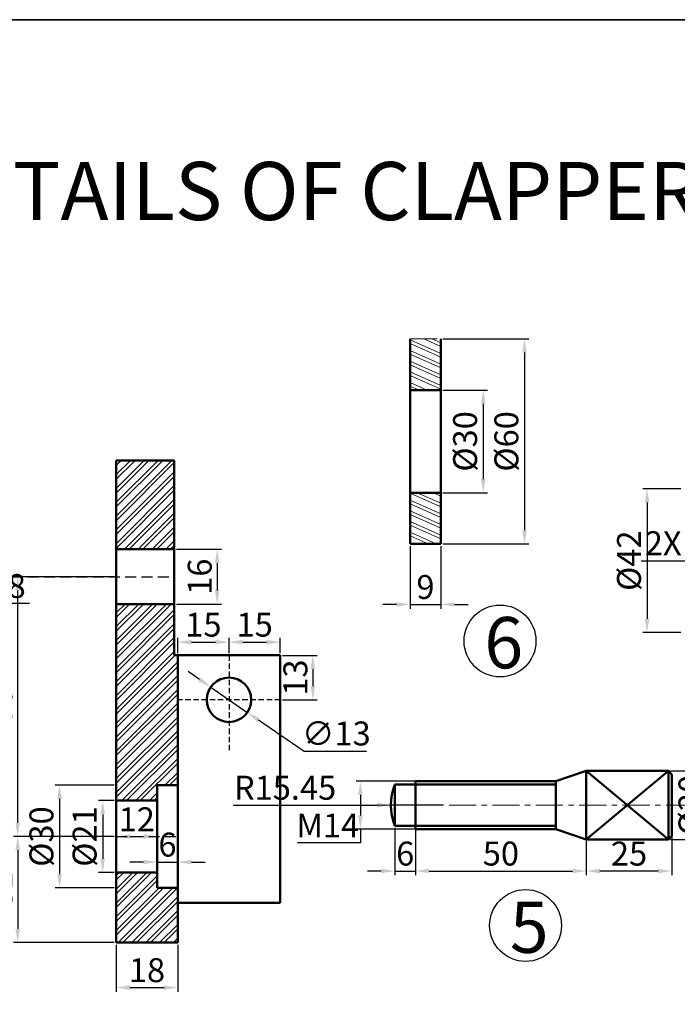
# Model space of a CAD drawing. Units: millimetres. Extents: x -108 to 732, y -172 to 297.
# Tile 3 of 4: x 91 to 284, y 9 to 297. Entities that reach past the tile are written whole.
import ezdxf

# ---------------------------------------------------------------- set-up
doc = ezdxf.new("R2010")
doc.units = ezdxf.units.MM
doc.header["$LTSCALE"] = 0.5
doc.linetypes.add('CENTER', pattern=[50.8, 31.75, -6.35, 6.35, -6.35])
doc.linetypes.add('HIDDEN', pattern=[9.525, 6.35, -3.175])
for name, color, linetype, lineweight in [('M-CNTR', 1, 'CENTER', 18), ('M-DIMS', 2, 'Continuous', 25), ('M-HATC', 8, 'Continuous', 18), ('M-HIDN', 6, 'HIDDEN', 25), ('M-OUTL', 7, 'Continuous', 50), ('M-SYMB', 3, 'Continuous', 25), ('M-TEXT', 3, 'Continuous', 25), ('M-TTLB', 7, 'Continuous', 35)]:
    doc.layers.add(name, color=color, linetype=linetype, lineweight=lineweight)
doc.styles.get("Standard").update_dxf_attribs({"font": 'arial.ttf'})
doc.dimstyles.new('ISO-25', dxfattribs={"dimtxt": 7, "dimasz": 4, "dimexe": 1.25, "dimexo": 0.625, "dimtad": 1, "dimtoh": 1, "dimtxsty": 'Standard', "dimcen": 2.5, "dimadec": 0, "dimazin": 0, "dimtfac": 1, "dimtmove": 0, "dimatfit": 3, "dimfxl": 1, "dimarcsym": 0})

# ---------------------------------------------------------------- blocks, each defined once
blk = doc.blocks.new('*D2')
at = {"layer": 'Defpoints', "color": 0, "ltscale": 0.5, "transparency": 16777216}
for p in [(119.6, 73.21), (103, 43.21), (119.6, 43.21)]:
    blk.add_point(p, dxfattribs=at)
at = {"layer": 'M-DIMS', "color": 0, "lineweight": -2, "ltscale": 0.5, "transparency": 16777216}
for p, q in [((118.97, 73.21), (101.75, 73.21)), ((103, 69.21), (103, 47.21)), ((118.97, 43.21), (101.75, 43.21))]:
    blk.add_line(p, q, dxfattribs=at)
at = {"layer": 'M-DIMS', "color": 0, "ltscale": 0.5, "transparency": 16777216}
for points in [[(102.33, 69.21), (103.67, 69.21), (103, 73.21)], [(102.33, 47.21), (103.67, 47.21), (103, 43.21)]]:
    blk.add_solid(points, dxfattribs=at)
at = {"layer": 'M-DIMS', "color": 0, "ltscale": 0.5, "transparency": 16777216, "insert": (98.61, 58.21), "char_height": 7, "attachment_point": 5, "rotation": 90}
blk.add_mtext('%%C30', dxfattribs=at)
blk = doc.blocks.new('*D3')
at = {"layer": 'Defpoints', "color": 0, "ltscale": 0.5, "transparency": 16777216}
for p in [(119.6, 68.71), (115.64, 47.71), (119.6, 47.71)]:
    blk.add_point(p, dxfattribs=at)
at = {"layer": 'M-DIMS', "color": 0, "lineweight": -2, "ltscale": 0.5, "transparency": 16777216}
for p, q in [((118.97, 68.71), (114.39, 68.71)), ((115.64, 64.71), (115.64, 51.71)), ((118.97, 47.71), (114.39, 47.71))]:
    blk.add_line(p, q, dxfattribs=at)
at = {"layer": 'M-DIMS', "color": 0, "ltscale": 0.5, "transparency": 16777216}
for points in [[(114.97, 64.71), (116.31, 64.71), (115.64, 68.71)], [(114.97, 51.71), (116.31, 51.71), (115.64, 47.71)]]:
    blk.add_solid(points, dxfattribs=at)
at = {"layer": 'M-DIMS', "color": 0, "ltscale": 0.5, "transparency": 16777216, "insert": (111.25, 58.21), "char_height": 7, "attachment_point": 5, "rotation": 90}
blk.add_mtext('%%C21', dxfattribs=at)
blk = doc.blocks.new('*D4')
at = {"layer": 'Defpoints', "color": 0, "ltscale": 0.5, "transparency": 16777216}
for p in [(152.6, 115.08), (137.6, 111.21), (152.6, 111.21)]:
    blk.add_point(p, dxfattribs=at)
at = {"layer": 'M-DIMS', "color": 0, "lineweight": -2, "ltscale": 0.5, "transparency": 16777216}
for p, q in [((137.6, 111.84), (137.6, 116.33)), ((152.6, 111.84), (152.6, 116.33)), ((141.6, 115.08), (148.6, 115.08))]:
    blk.add_line(p, q, dxfattribs=at)
at = {"layer": 'M-DIMS', "color": 0, "ltscale": 0.5, "transparency": 16777216}
for points in [[(141.6, 115.75), (141.6, 114.41), (137.6, 115.08)], [(148.6, 115.75), (148.6, 114.41), (152.6, 115.08)]]:
    blk.add_solid(points, dxfattribs=at)
at = {"layer": 'M-DIMS', "color": 0, "ltscale": 0.5, "transparency": 16777216, "insert": (145.1, 119.28), "char_height": 7, "attachment_point": 5}
blk.add_mtext('15', dxfattribs=at)
blk = doc.blocks.new('*D5')
at = {"layer": 'Defpoints', "color": 0, "ltscale": 0.5, "transparency": 16777216}
for p in [(167.6, 115.08), (152.6, 111.21), (167.6, 111.21)]:
    blk.add_point(p, dxfattribs=at)
at = {"layer": 'M-DIMS', "color": 0, "lineweight": -2, "ltscale": 0.5, "transparency": 16777216}
for p, q in [((152.6, 111.84), (152.6, 116.33)), ((167.6, 111.84), (167.6, 116.33)), ((156.6, 115.08), (163.6, 115.08))]:
    blk.add_line(p, q, dxfattribs=at)
at = {"layer": 'M-DIMS', "color": 0, "ltscale": 0.5, "transparency": 16777216}
for points in [[(156.6, 115.75), (156.6, 114.41), (152.6, 115.08)], [(163.6, 115.75), (163.6, 114.41), (167.6, 115.08)]]:
    blk.add_solid(points, dxfattribs=at)
at = {"layer": 'M-DIMS', "color": 0, "ltscale": 0.5, "transparency": 16777216, "insert": (160.1, 119.28), "char_height": 7, "attachment_point": 5}
blk.add_mtext('15', dxfattribs=at)
blk = doc.blocks.new('*D6')
at = {"layer": 'Defpoints', "color": 0, "ltscale": 0.5, "transparency": 16777216}
for p in [(167.6, 111.21), (167.6, 98.21), (177.13, 98.21)]:
    blk.add_point(p, dxfattribs=at)
at = {"layer": 'M-DIMS', "color": 0, "lineweight": -2, "ltscale": 0.5, "transparency": 16777216}
for p, q in [((168.22, 111.21), (178.38, 111.21)), ((177.13, 107.21), (177.13, 102.21)), ((168.22, 98.21), (178.38, 98.21))]:
    blk.add_line(p, q, dxfattribs=at)
at = {"layer": 'M-DIMS', "color": 0, "ltscale": 0.5, "transparency": 16777216}
for points in [[(176.46, 107.21), (177.8, 107.21), (177.13, 111.21)], [(176.46, 102.21), (177.8, 102.21), (177.13, 98.21)]]:
    blk.add_solid(points, dxfattribs=at)
at = {"layer": 'M-DIMS', "color": 0, "ltscale": 0.5, "transparency": 16777216, "insert": (172.93, 104.71), "char_height": 7, "attachment_point": 5, "rotation": 90}
blk.add_mtext('13', dxfattribs=at)
blk = doc.blocks.new('*D7')
at = {"layer": 'Defpoints', "color": 0, "ltscale": 0.5, "transparency": 16777216}
for p in [(119.6, 27.21), (137.6, 27.21), (137.6, 14.04)]:
    blk.add_point(p, dxfattribs=at)
at = {"layer": 'M-DIMS', "color": 0, "lineweight": -2, "ltscale": 0.5, "transparency": 16777216}
for p, q in [((119.6, 26.59), (119.6, 12.79)), ((137.6, 26.59), (137.6, 12.79)), ((123.6, 14.04), (133.6, 14.04))]:
    blk.add_line(p, q, dxfattribs=at)
at = {"layer": 'M-DIMS', "color": 0, "ltscale": 0.5, "transparency": 16777216}
for points in [[(123.6, 14.7), (123.6, 13.37), (119.6, 14.04)], [(133.6, 14.7), (133.6, 13.37), (137.6, 14.04)]]:
    blk.add_solid(points, dxfattribs=at)
at = {"layer": 'M-DIMS', "color": 0, "ltscale": 0.5, "transparency": 16777216, "insert": (128.6, 18.24), "char_height": 7, "attachment_point": 5}
blk.add_mtext('18', dxfattribs=at)
blk = doc.blocks.new('*D8')
at = {"layer": 'Defpoints', "color": 0, "ltscale": 0.5, "transparency": 16777216}
for p in [(137.6, 50.75), (131.6, 43.21), (137.6, 43.21)]:
    blk.add_point(p, dxfattribs=at)
at = {"layer": 'M-DIMS', "color": 0, "lineweight": -2, "ltscale": 0.5, "transparency": 16777216}
for p, q in [((131.6, 43.84), (131.6, 52)), ((137.6, 43.84), (137.6, 52)), ((127.6, 50.75), (123.6, 50.75)), ((131.6, 50.75), (137.6, 50.75)), ((141.6, 50.75), (145.6, 50.75))]:
    blk.add_line(p, q, dxfattribs=at)
at = {"layer": 'M-DIMS', "color": 0, "ltscale": 0.5, "transparency": 16777216}
for points in [[(127.6, 51.42), (127.6, 50.09), (131.6, 50.75)], [(141.6, 51.42), (141.6, 50.09), (137.6, 50.75)]]:
    blk.add_solid(points, dxfattribs=at)
at = {"layer": 'M-DIMS', "color": 0, "ltscale": 0.5, "transparency": 16777216, "insert": (134.6, 54.95), "char_height": 7, "attachment_point": 5}
blk.add_mtext('6', dxfattribs=at)
blk = doc.blocks.new('*D9')
at = {"layer": 'Defpoints', "color": 0, "ltscale": 0.5, "transparency": 16777216}
for p in [(119.6, 58.21), (90.76, 27.21), (119.6, 27.21)]:
    blk.add_point(p, dxfattribs=at)
at = {"layer": 'M-DIMS', "color": 0, "lineweight": -2, "ltscale": 0.5, "transparency": 16777216}
for p, q in [((118.97, 58.21), (89.51, 58.21)), ((90.76, 54.21), (90.76, 31.21)), ((118.97, 27.21), (89.51, 27.21))]:
    blk.add_line(p, q, dxfattribs=at)
at = {"layer": 'M-DIMS', "color": 0, "ltscale": 0.5, "transparency": 16777216}
for points in [[(90.09, 54.21), (91.43, 54.21), (90.76, 58.21)], [(90.09, 31.21), (91.43, 31.21), (90.76, 27.21)]]:
    blk.add_solid(points, dxfattribs=at)
at = {"layer": 'M-DIMS', "color": 0, "ltscale": 0.5, "transparency": 16777216, "insert": (86.56, 42.71), "char_height": 7, "attachment_point": 5, "rotation": 90}
blk.add_mtext('31', dxfattribs=at)
blk = doc.blocks.new('*D10')
at = {"layer": 'Defpoints', "color": 0, "ltscale": 0.5, "transparency": 16777216}
for p in [(90.76, 134.21), (119.6, 134.21), (90.76, 58.21)]:
    blk.add_point(p, dxfattribs=at)
at = {"layer": 'M-DIMS', "color": 0, "lineweight": -2, "ltscale": 0.5, "transparency": 16777216}
for p, q in [((118.97, 134.21), (89.51, 134.21)), ((90.76, 62.21), (90.76, 130.21)), ((90.14, 58.21), (89.51, 58.21))]:
    blk.add_line(p, q, dxfattribs=at)
at = {"layer": 'M-DIMS', "color": 0, "ltscale": 0.5, "transparency": 16777216}
for points in [[(90.09, 130.21), (91.43, 130.21), (90.76, 134.21)], [(90.09, 62.21), (91.43, 62.21), (90.76, 58.21)]]:
    blk.add_solid(points, dxfattribs=at)
at = {"layer": 'M-DIMS', "color": 0, "ltscale": 0.5, "transparency": 16777216, "insert": (86.56, 96.21), "char_height": 7, "attachment_point": 5, "rotation": 90}
blk.add_mtext('76', dxfattribs=at)
blk = doc.blocks.new('*D11')
at = {"layer": 'Defpoints', "color": 0, "ltscale": 0.5, "transparency": 16777216}
for p in [(147.25, 101.91), (157.95, 94.52)]:
    blk.add_point(p, dxfattribs=at)
at = {"layer": 'M-DIMS', "color": 0, "lineweight": -2, "ltscale": 0.5, "transparency": 16777216}
for p, q in [((143.96, 104.18), (140.67, 106.46)), ((147.25, 101.91), (157.95, 94.52)), ((174.55, 83.06), (161.24, 92.25)), ((192.81, 83.06), (174.55, 83.06))]:
    blk.add_line(p, q, dxfattribs=at)
at = {"layer": 'M-DIMS', "color": 0, "ltscale": 0.5, "transparency": 16777216}
for points in [[(144.34, 104.73), (143.58, 103.63), (147.25, 101.91)], [(161.62, 92.8), (160.86, 91.7), (157.95, 94.52)]]:
    blk.add_solid(points, dxfattribs=at)
at = {"layer": 'M-DIMS', "color": 0, "ltscale": 0.5, "transparency": 16777216, "insert": (183.99, 87.45), "char_height": 7, "attachment_point": 5}
blk.add_mtext('∅13', dxfattribs=at)
blk = doc.blocks.new('*D12')
at = {"layer": 'Defpoints', "color": 0, "ltscale": 0.5, "transparency": 16777216}
for p in [(136.6, 142.21), (136.6, 126.21), (149.14, 126.21)]:
    blk.add_point(p, dxfattribs=at)
at = {"layer": 'M-DIMS', "color": 0, "lineweight": -2, "ltscale": 0.5, "transparency": 16777216}
for p, q in [((137.22, 142.21), (150.39, 142.21)), ((149.14, 138.21), (149.14, 130.21)), ((137.22, 126.21), (150.39, 126.21))]:
    blk.add_line(p, q, dxfattribs=at)
at = {"layer": 'M-DIMS', "color": 0, "ltscale": 0.5, "transparency": 16777216}
for points in [[(148.47, 138.21), (149.8, 138.21), (149.14, 142.21)], [(148.47, 130.21), (149.8, 130.21), (149.14, 126.21)]]:
    blk.add_solid(points, dxfattribs=at)
at = {"layer": 'M-DIMS', "color": 0, "ltscale": 0.5, "transparency": 16777216, "insert": (144.94, 134.21), "char_height": 7, "attachment_point": 5, "rotation": 90}
blk.add_mtext('16', dxfattribs=at)
blk = doc.blocks.new('*D13')
at = {"layer": 'Defpoints', "color": 0, "ltscale": 0.5, "transparency": 16777216}
for p in [(119.6, 62.33), (131.6, 62.33), (131.6, 58.21)]:
    blk.add_point(p, dxfattribs=at)
at = {"layer": 'M-DIMS', "color": 0, "lineweight": -2, "ltscale": 0.5, "transparency": 16777216}
for p, q in [((119.6, 61.71), (119.6, 56.96)), ((131.6, 61.71), (131.6, 56.96)), ((123.6, 58.21), (127.6, 58.21))]:
    blk.add_line(p, q, dxfattribs=at)
at = {"layer": 'M-DIMS', "color": 0, "ltscale": 0.5, "transparency": 16777216}
for points in [[(123.6, 58.88), (123.6, 57.55), (119.6, 58.21)], [(127.6, 58.88), (127.6, 57.55), (131.6, 58.21)]]:
    blk.add_solid(points, dxfattribs=at)
at = {"layer": 'M-DIMS', "color": 0, "ltscale": 0.5, "transparency": 16777216, "insert": (125.6, 62.35), "char_height": 7, "attachment_point": 5}
blk.add_mtext('12', dxfattribs=at)
blk = doc.blocks.new('*D34')
at = {"layer": 'Defpoints', "color": 0, "ltscale": 0.5, "transparency": 16777216}
for p in [(214.58, 188.77), (214.58, 158.77), (226.99, 158.77)]:
    blk.add_point(p, dxfattribs=at)
at = {"layer": 'M-DIMS', "color": 0, "lineweight": -2, "ltscale": 0.5, "transparency": 16777216}
for p, q in [((215.2, 188.77), (228.24, 188.77)), ((226.99, 184.77), (226.99, 162.77)), ((215.2, 158.77), (228.24, 158.77))]:
    blk.add_line(p, q, dxfattribs=at)
at = {"layer": 'M-DIMS', "color": 0, "ltscale": 0.5, "transparency": 16777216}
for points in [[(226.32, 184.77), (227.65, 184.77), (226.99, 188.77)], [(226.32, 162.77), (227.65, 162.77), (226.99, 158.77)]]:
    blk.add_solid(points, dxfattribs=at)
at = {"layer": 'M-DIMS', "color": 0, "ltscale": 0.5, "transparency": 16777216, "insert": (222.59, 173.77), "char_height": 7, "attachment_point": 5, "rotation": 90}
blk.add_mtext('%%C30', dxfattribs=at)
blk = doc.blocks.new('*D35')
at = {"layer": 'Defpoints', "color": 0, "ltscale": 0.5, "transparency": 16777216}
for p in [(214.58, 203.77), (214.58, 143.77), (239.06, 143.77)]:
    blk.add_point(p, dxfattribs=at)
at = {"layer": 'M-DIMS', "color": 0, "lineweight": -2, "ltscale": 0.5, "transparency": 16777216}
for p, q in [((215.2, 203.77), (240.31, 203.77)), ((239.06, 199.77), (239.06, 147.77)), ((215.2, 143.77), (240.31, 143.77))]:
    blk.add_line(p, q, dxfattribs=at)
at = {"layer": 'M-DIMS', "color": 0, "ltscale": 0.5, "transparency": 16777216}
for points in [[(238.4, 199.77), (239.73, 199.77), (239.06, 203.77)], [(238.4, 147.77), (239.73, 147.77), (239.06, 143.77)]]:
    blk.add_solid(points, dxfattribs=at)
at = {"layer": 'M-DIMS', "color": 0, "ltscale": 0.5, "transparency": 16777216, "insert": (234.67, 173.77), "char_height": 7, "attachment_point": 5, "rotation": 90}
blk.add_mtext('%%C60', dxfattribs=at)
blk = doc.blocks.new('*D36')
at = {"layer": 'Defpoints', "color": 0, "ltscale": 0.5, "transparency": 16777216}
for p in [(205.58, 143.77), (214.58, 143.77), (214.58, 126.1)]:
    blk.add_point(p, dxfattribs=at)
at = {"layer": 'M-DIMS', "color": 0, "lineweight": -2, "ltscale": 0.5, "transparency": 16777216}
for p, q in [((205.58, 143.15), (205.58, 124.85)), ((214.58, 143.15), (214.58, 124.85)), ((201.58, 126.1), (197.58, 126.1)), ((205.58, 126.1), (214.58, 126.1)), ((218.58, 126.1), (222.58, 126.1))]:
    blk.add_line(p, q, dxfattribs=at)
at = {"layer": 'M-DIMS', "color": 0, "ltscale": 0.5, "transparency": 16777216}
for points in [[(201.58, 126.76), (201.58, 125.43), (205.58, 126.1)], [(218.58, 126.76), (218.58, 125.43), (214.58, 126.1)]]:
    blk.add_solid(points, dxfattribs=at)
at = {"layer": 'M-DIMS', "color": 0, "ltscale": 0.5, "transparency": 16777216, "insert": (210.08, 130.29), "char_height": 7, "attachment_point": 5}
blk.add_mtext('9', dxfattribs=at)
blk = doc.blocks.new('*D37')
at = {"layer": 'Defpoints', "color": 0, "ltscale": 0.5, "transparency": 16777216}
for p in [(201.16, 61.4), (207.16, 61.4), (207.16, 48.13)]:
    blk.add_point(p, dxfattribs=at)
at = {"layer": 'M-DIMS', "color": 0, "lineweight": -2, "ltscale": 0.5, "transparency": 16777216}
for p, q in [((201.16, 60.77), (201.16, 46.88)), ((207.16, 60.77), (207.16, 46.88)), ((197.16, 48.13), (193.16, 48.13)), ((201.16, 48.13), (207.16, 48.13)), ((211.16, 48.13), (215.16, 48.13))]:
    blk.add_line(p, q, dxfattribs=at)
at = {"layer": 'M-DIMS', "color": 0, "ltscale": 0.5, "transparency": 16777216}
for points in [[(197.16, 48.8), (197.16, 47.47), (201.16, 48.13)], [(211.16, 48.8), (211.16, 47.47), (207.16, 48.13)]]:
    blk.add_solid(points, dxfattribs=at)
at = {"layer": 'M-DIMS', "color": 0, "ltscale": 0.5, "transparency": 16777216, "insert": (204.16, 52.33), "char_height": 7, "attachment_point": 5}
blk.add_mtext('6', dxfattribs=at)
blk = doc.blocks.new('*D38')
at = {"layer": 'Defpoints', "color": 0, "ltscale": 0.5, "transparency": 16777216}
for p in [(207.16, 67.4), (257.16, 67.4), (257.16, 48.13)]:
    blk.add_point(p, dxfattribs=at)
at = {"layer": 'M-DIMS', "color": 0, "lineweight": -2, "ltscale": 0.5, "transparency": 16777216}
for p, q in [((207.16, 66.77), (207.16, 46.88)), ((257.16, 66.77), (257.16, 46.88)), ((211.16, 48.13), (253.16, 48.13))]:
    blk.add_line(p, q, dxfattribs=at)
at = {"layer": 'M-DIMS', "color": 0, "ltscale": 0.5, "transparency": 16777216}
for points in [[(211.16, 48.8), (211.16, 47.47), (207.16, 48.13)], [(253.16, 48.8), (253.16, 47.47), (257.16, 48.13)]]:
    blk.add_solid(points, dxfattribs=at)
at = {"layer": 'M-DIMS', "color": 0, "ltscale": 0.5, "transparency": 16777216, "insert": (232.16, 52.33), "char_height": 7, "attachment_point": 5}
blk.add_mtext('50', dxfattribs=at)
blk = doc.blocks.new('*D39')
at = {"layer": 'Defpoints', "color": 0, "ltscale": 0.5, "transparency": 16777216}
for p in [(257.16, 67.4), (282.16, 67.4), (257.16, 48.13)]:
    blk.add_point(p, dxfattribs=at)
at = {"layer": 'M-DIMS', "color": 0, "lineweight": -2, "ltscale": 0.5, "transparency": 16777216}
for p, q in [((257.16, 66.77), (257.16, 46.88)), ((282.16, 66.77), (282.16, 46.88)), ((278.16, 48.13), (261.16, 48.13))]:
    blk.add_line(p, q, dxfattribs=at)
at = {"layer": 'M-DIMS', "color": 0, "ltscale": 0.5, "transparency": 16777216}
for points in [[(261.16, 48.8), (261.16, 47.47), (257.16, 48.13)], [(278.16, 48.8), (278.16, 47.47), (282.16, 48.13)]]:
    blk.add_solid(points, dxfattribs=at)
at = {"layer": 'M-DIMS', "color": 0, "ltscale": 0.5, "transparency": 16777216, "insert": (269.66, 52.33), "char_height": 7, "attachment_point": 5}
blk.add_mtext('25', dxfattribs=at)
blk = doc.blocks.new('*D40')
at = {"layer": 'Defpoints', "color": 0, "ltscale": 0.5, "transparency": 16777216}
for p in [(281.16, 77.4), (281.16, 57.4), (292.93, 57.4)]:
    blk.add_point(p, dxfattribs=at)
at = {"layer": 'M-DIMS', "color": 0, "lineweight": -2, "ltscale": 0.5, "transparency": 16777216}
for p, q in [((281.79, 77.4), (294.18, 77.4)), ((292.93, 73.4), (292.93, 61.4)), ((281.79, 57.4), (294.18, 57.4))]:
    blk.add_line(p, q, dxfattribs=at)
at = {"layer": 'M-DIMS', "color": 0, "ltscale": 0.5, "transparency": 16777216}
for points in [[(292.26, 73.4), (293.59, 73.4), (292.93, 77.4)], [(292.26, 61.4), (293.59, 61.4), (292.93, 57.4)]]:
    blk.add_solid(points, dxfattribs=at)
at = {"layer": 'M-DIMS', "color": 0, "ltscale": 0.5, "transparency": 16777216, "insert": (288.53, 67.4), "char_height": 7, "attachment_point": 5, "rotation": 90}
blk.add_mtext('%%C20', dxfattribs=at)
blk = doc.blocks.new('*D41')
at = {"layer": 'Defpoints', "color": 0, "ltscale": 0.5, "transparency": 16777216}
for p in [(212.85, 74.4), (191.05, 60.4), (212.85, 60.4)]:
    blk.add_point(p, dxfattribs=at)
at = {"layer": 'M-DIMS', "color": 0, "lineweight": -2, "ltscale": 0.5, "transparency": 16777216}
for p, q in [((212.23, 74.4), (189.8, 74.4)), ((191.05, 70.4), (191.05, 64.4)), ((212.23, 60.4), (189.8, 60.4)), ((191.05, 60.4), (191.05, 56.4)), ((191.05, 56.4), (172.6, 56.4))]:
    blk.add_line(p, q, dxfattribs=at)
at = {"layer": 'M-DIMS', "color": 0, "ltscale": 0.5, "transparency": 16777216}
for points in [[(190.38, 70.4), (191.71, 70.4), (191.05, 74.4)], [(190.38, 64.4), (191.71, 64.4), (191.05, 60.4)]]:
    blk.add_solid(points, dxfattribs=at)
at = {"layer": 'M-DIMS', "color": 0, "ltscale": 0.5, "transparency": 16777216, "insert": (181.51, 60.54), "char_height": 7, "attachment_point": 5}
blk.add_mtext('M14', dxfattribs=at)
blk = doc.blocks.new('*D46')
at = {"layer": 'Defpoints', "color": 0, "ltscale": 0.5, "transparency": 16777216}
for p in [(285.41, 159.89), (274.94, 117.89), (285.41, 117.89)]:
    blk.add_point(p, dxfattribs=at)
at = {"layer": 'M-DIMS', "color": 0, "lineweight": -2, "ltscale": 0.5, "transparency": 16777216}
for p, q in [((284.79, 159.89), (273.69, 159.89)), ((274.94, 155.89), (274.94, 121.89)), ((284.79, 117.89), (273.69, 117.89))]:
    blk.add_line(p, q, dxfattribs=at)
at = {"layer": 'M-DIMS', "color": 0, "ltscale": 0.5, "transparency": 16777216}
for points in [[(274.28, 155.89), (275.61, 155.89), (274.94, 159.89)], [(274.28, 121.89), (275.61, 121.89), (274.94, 117.89)]]:
    blk.add_solid(points, dxfattribs=at)
at = {"layer": 'M-DIMS', "color": 0, "ltscale": 0.5, "transparency": 16777216, "insert": (270.55, 138.89), "char_height": 7, "attachment_point": 5, "rotation": 90}
blk.add_mtext('%%C42', dxfattribs=at)
blk = doc.blocks.new('*D54')
at = {"layer": 'Defpoints', "color": 0, "ltscale": 0.5, "transparency": 16777216}
for p in [(45.34, 134.21), (52.87, 131.51)]:
    blk.add_point(p, dxfattribs=at)
at = {"layer": 'M-DIMS', "color": 0, "lineweight": -2, "ltscale": 0.5, "transparency": 16777216}
for p, q in [((45.34, 134.21), (52.87, 131.51)), ((67.12, 126.38), (56.63, 130.15)), ((94.21, 126.38), (67.12, 126.38))]:
    blk.add_line(p, q, dxfattribs=at)
at = {"layer": 'M-DIMS', "color": 0, "ltscale": 0.5, "transparency": 16777216}
blk.add_solid([(56.86, 130.78), (56.41, 129.53), (52.87, 131.51)], dxfattribs=at)
at = {"layer": 'M-DIMS', "color": 0, "ltscale": 0.5, "transparency": 16777216, "insert": (80.98, 130.58), "char_height": 7, "attachment_point": 5}
blk.add_mtext('2X R8', dxfattribs=at)
blk = doc.blocks.new('*D59')
at = {"layer": 'Defpoints', "color": 0, "ltscale": 0.5, "transparency": 16777216}
for p in [(315.41, 138.89), (324.41, 138.89)]:
    blk.add_point(p, dxfattribs=at)
at = {"layer": 'M-DIMS', "color": 0, "lineweight": -2, "ltscale": 0.5, "transparency": 16777216}
for p, q in [((273.18, 138.89), (300.26, 138.89)), ((300.26, 138.89), (311.41, 138.89)), ((324.41, 138.89), (315.41, 138.89))]:
    blk.add_line(p, q, dxfattribs=at)
at = {"layer": 'M-DIMS', "color": 0, "ltscale": 0.5, "transparency": 16777216}
blk.add_solid([(311.41, 139.56), (311.41, 138.23), (315.41, 138.89)], dxfattribs=at)
at = {"layer": 'M-DIMS', "color": 0, "ltscale": 0.5, "transparency": 16777216, "insert": (286.41, 143.09), "char_height": 7, "attachment_point": 5}
blk.add_mtext('2X R9', dxfattribs=at)
blk = doc.blocks.new('*D60')
at = {"layer": 'Defpoints', "color": 0, "ltscale": 0.5, "transparency": 16777216}
for p in [(199.95, 67.4), (215.4, 67.4)]:
    blk.add_point(p, dxfattribs=at)
at = {"layer": 'M-DIMS', "color": 0, "lineweight": -2, "ltscale": 0.5, "transparency": 16777216}
for p, q in [((153.8, 67.4), (184.8, 67.4)), ((184.8, 67.4), (195.95, 67.4)), ((215.4, 67.4), (199.95, 67.4))]:
    blk.add_line(p, q, dxfattribs=at)
at = {"layer": 'M-DIMS', "color": 0, "ltscale": 0.5, "transparency": 16777216}
blk.add_solid([(195.95, 68.06), (195.95, 66.73), (199.95, 67.4)], dxfattribs=at)
at = {"layer": 'M-DIMS', "color": 0, "ltscale": 0.5, "transparency": 16777216, "insert": (168.99, 71.59), "char_height": 7, "attachment_point": 5}
blk.add_mtext('R15.45', dxfattribs=at)

msp = doc.modelspace()

# ---------------------------------------------------------------- hatches: boundary and pattern name
at = {"layer": 'M-HATC', "ltscale": 0.5}
h = msp.add_hatch(dxfattribs=at)
h.set_pattern_fill('ANSI32', color=256, scale=0.3, angle=111)
h.set_pattern_definition([(156, (-22.2835, 81.8146), (-1.16225, -2.610456), []), (156, (-22.7662, 83.0722), (-1.16225, -2.610456), [])])
h.paths.add_polyline_path([(205.578, 188.772), (214.578, 188.772), (214.578, 203.772), (205.578, 203.772)])
h.paths.add_polyline_path([(205.578, 143.772), (214.578, 143.772), (214.578, 158.772), (205.578, 158.772)])
h = msp.add_hatch(dxfattribs=at)
h.set_pattern_fill('ANSI32', color=256, scale=0.3)
h.paths.add_polyline_path([(136.598, 168.214), (119.598, 168.214), (119.598, 142.214), (136.598, 142.214)])
h = msp.add_hatch(dxfattribs=at)
h.set_pattern_fill('ANSI32', color=256, scale=0.3)
h.paths.add_polyline_path([(137.598, 43.214), (131.598, 43.214), (131.598, 47.714), (119.598, 47.714), (119.598, 27.214), (137.598, 27.214)])
h.paths.add_polyline_path([(137.598, 111.214), (136.598, 111.214), (136.598, 126.214), (119.598, 126.214), (119.598, 68.714), (131.598, 68.714), (131.598, 73.214), (137.598, 73.214)])

# ---------------------------------------------------------------- linework, layer by layer
at = {"layer": 'M-CNTR', "ltscale": 0.5}
for p, q in [((205.578, 203.772), (214.578, 203.772)), ((288.425, 67.396), (190.313, 67.396))]:
    msp.add_line(p, q, dxfattribs=at)
at = {"layer": 'M-HIDN', "ltscale": 0.5}
for p, q in [((276.384, 138.892), (401.359, 138.892)), ((152.598, 111.214), (152.598, 83.055)), ((167.598, 98.214), (137.598, 98.214))]:
    msp.add_line(p, q, dxfattribs=at)
at = {"layer": 'M-HIDN'}
for p, q in [((-30.16, 134.214), (136.598, 134.214)), ((119.598, 58.214), (137.598, 58.214))]:
    msp.add_line(p, q, dxfattribs=at)
at = {"layer": 'M-OUTL', "ltscale": 0.5}
for p, q in [((205.578, 143.772), (205.578, 203.772)), ((214.578, 203.772), (214.578, 143.772)), ((214.578, 188.772), (205.578, 188.772)), ((214.578, 158.772), (205.578, 158.772)), ((214.578, 143.772), (205.578, 143.772)), ((167.598, 38.838), (167.598, 98.214)), ((248.242, 74.396), (257.161, 77.396)), ((257.161, 77.396), (281.161, 77.396)), ((257.161, 57.396), (257.161, 77.396)), ((281.161, 57.396), (257.161, 77.396)), ((257.161, 57.396), (281.161, 77.396)), ((281.161, 77.396), (281.161, 57.396)), ((281.161, 77.396), (282.161, 76.396)), ((282.161, 76.396), (282.161, 58.396)), ((201.161, 61.396), (201.161, 73.396)), ((248.242, 73.396), (201.161, 73.396)), ((207.161, 60.396), (207.161, 74.396)), ((248.242, 74.396), (207.161, 74.396)), ((248.242, 74.396), (248.242, 60.396)), ((248.242, 61.396), (201.161, 61.396)), ((248.242, 60.396), (207.161, 60.396)), ((248.242, 60.396), (257.161, 57.396)), ((281.161, 57.396), (282.161, 58.396)), ((281.161, 57.396), (257.161, 57.396)), ((137.598, 38.838), (167.598, 38.838))]:
    msp.add_line(p, q, dxfattribs=at)
at = {"layer": 'M-OUTL'}
for p, q in [((119.598, 168.214), (119.598, 27.214)), ((119.598, 168.214), (136.598, 168.214)), ((136.598, 168.214), (136.598, 111.214)), ((119.598, 142.214), (136.598, 142.214)), ((119.598, 126.214), (136.598, 126.214)), ((136.598, 111.214), (137.598, 111.214)), ((137.598, 27.214), (137.598, 111.214)), ((137.598, 111.214), (152.598, 111.214)), ((152.598, 111.214), (167.598, 111.214)), ((167.598, 111.214), (167.598, 98.214)), ((131.598, 73.214), (131.598, 43.214)), ((131.598, 73.214), (137.598, 73.214)), ((119.598, 68.714), (131.598, 68.714)), ((119.598, 68.714), (119.598, 47.714)), ((119.598, 47.714), (131.598, 47.714)), ((131.598, 43.214), (137.598, 43.214)), ((119.598, 27.214), (137.598, 27.214))]:
    msp.add_line(p, q, dxfattribs=at)
msp.add_circle((152.598, 98.214), 6.5, dxfattribs=at)
at = {"layer": 'M-OUTL', "ltscale": 0.5}
msp.add_arc((215.399, 67.396), 15.451, 157.14951, 202.85049, dxfattribs=at)
at = {"layer": 'M-SYMB', "ltscale": 0.5}
for centre in [(231.917, 115.403), (239.384, 32.204)]:
    msp.add_circle(centre, 10.513, dxfattribs=at)
at = {"layer": 'M-TTLB', "ltscale": 0.5}
msp.add_lwpolyline([(-108.335, 297.096), (732.37, 297.096), (732.37, -172.452), (-108.335, -172.452)], close=True, dxfattribs=at)

# ---------------------------------------------------------------- texts
at = {"layer": 'M-TEXT', "ltscale": 0.5, "attachment_point": 1}
for s, width, heights, insert, char_height in [('\\pxqc;DETAILS OF CLAPPER BLOCK', 372.02553, [0], (28.998, 255.491), 17), ('6', 20, [1.225], (227.314, 122.411), 15), ('5', 20, [1.225], (234.781, 39.213), 15)]:
    msp.add_mtext_dynamic_manual_height_columns(s, width=width, gutter_width=12.5, heights=heights, dxfattribs=dict(at, insert=insert, char_height=char_height))

# ---------------------------------------------------------------- dimensions: what is measured, and where the dimension line sits
at = {"layer": 'M-DIMS', "ltscale": 0.5}
for base, p1, p2, text, picture, middle in [((239.065, 143.772), (214.578, 203.772), (214.578, 143.772), '%%C<>', '*D35', (234.67, 173.772)), ((226.987, 158.772), (214.578, 188.772), (214.578, 158.772), '%%C<>', '*D34', (222.592, 173.772)), ((274.945, 117.892), (285.412, 159.892), (285.412, 117.892), '%%C<>', '*D46', (270.55, 138.892)), ((292.927, 57.396), (281.161, 77.396), (281.161, 57.396), '%%C<>', '*D40', (288.533, 67.396)), ((103.001, 43.214), (119.598, 73.214), (119.598, 43.214), '%%C<>', '*D2', (98.606, 58.214)), ((191.047, 60.396), (212.854, 74.396), (212.854, 60.396), 'M<>', '*D41', (181.509, 60.536)), ((115.641, 47.714), (119.598, 68.714), (119.598, 47.714), '%%C<>', '*D3', (111.247, 58.214))]:
    dim = msp.add_linear_dim(base=base, p1=p1, p2=p2, angle=90, text=text, dimstyle='ISO-25', override={"dimclrd": 0, "dimclre": 0, "dimclrt": 0}, dxfattribs=at)
    dim.commit()
    dim.dimension.update_dxf_attribs({"geometry": picture, "text_midpoint": middle})
for center, mpoint, picture, middle in [((324.412, 138.892), (315.412, 138.892), '*D59', (286.408, 143.09)), ((45.34, 134.214), (52.869, 131.508), '*D54', (80.98, 130.582))]:
    dim = msp.add_radius_dim(center=center, mpoint=mpoint, text='2X <>', dimstyle='ISO-25', override={"dimdec": 0, "dimlfac": 1, "dimrnd": 0, "dimzin": 0, "dimdsep": 46, "dimlunit": 2}, dxfattribs=at)
    dim.commit()
    dim.dimension.update_dxf_attribs({"geometry": picture, "text_midpoint": middle})
for base, p1, p2, picture, middle in [((149.135, 126.214), (136.598, 142.214), (136.598, 126.214), '*D12', (144.936, 134.214)), ((90.761, 134.214), (90.761, 58.214), (119.598, 134.214), '*D10', (86.562, 96.214)), ((177.13, 98.214), (167.598, 111.214), (167.598, 98.214), '*D6', (172.928, 104.714)), ((90.761, 27.214), (119.598, 58.214), (119.598, 27.214), '*D9', (86.559, 42.714))]:
    dim = msp.add_linear_dim(base=base, p1=p1, p2=p2, angle=90, dimstyle='ISO-25', override={"dimclrd": 0, "dimclre": 0, "dimclrt": 0}, dxfattribs=at)
    dim.commit()
    dim.dimension.update_dxf_attribs({"geometry": picture, "text_midpoint": middle})
for base, p1, p2, picture, middle in [((214.578, 126.096), (205.578, 143.772), (214.578, 143.772), '*D36', (210.078, 130.295)), ((152.598, 115.079), (137.598, 111.214), (152.598, 111.214), '*D4', (145.098, 119.278)), ((167.598, 115.079), (152.598, 111.214), (167.598, 111.214), '*D5', (160.098, 119.278)), ((131.598, 58.214), (119.598, 62.331), (131.598, 62.331), '*D13', (125.598, 62.354)), ((257.161, 48.133), (207.161, 67.396), (257.161, 67.396), '*D38', (232.161, 52.332)), ((257.161, 48.133), (282.161, 67.396), (257.161, 67.396), '*D39', (269.661, 52.332)), ((207.161, 48.133), (201.161, 61.396), (207.161, 61.396), '*D37', (204.161, 52.332)), ((137.598, 50.752), (131.598, 43.214), (137.598, 43.214), '*D8', (134.598, 54.951)), ((137.598, 14.038), (119.598, 27.214), (137.598, 27.214), '*D7', (128.598, 18.237))]:
    dim = msp.add_linear_dim(base=base, p1=p1, p2=p2, dimstyle='ISO-25', override={"dimclrd": 0, "dimclre": 0, "dimclrt": 0}, dxfattribs=at)
    dim.commit()
    dim.dimension.update_dxf_attribs({"geometry": picture, "text_midpoint": middle})
dim = msp.add_diameter_dim_2p(p1=(147.25, 101.909), p2=(157.947, 94.52), dimstyle='ISO-25', override={"dimclrd": 0, "dimclre": 0, "dimclrt": 0}, dxfattribs=at)
dim.commit()
dim.dimension.update_dxf_attribs({"geometry": '*D11', "text_midpoint": (183.992, 83.055), "dimtype": 163})
dim = msp.add_radius_dim(center=(215.399, 67.396), mpoint=(199.948, 67.396), dimstyle='ISO-25', override={"dimdec": 2, "dimlfac": 1, "dimrnd": 0, "dimzin": 0, "dimdsep": 46, "dimlunit": 2}, dxfattribs=at)
dim.commit()
dim.dimension.update_dxf_attribs({"geometry": '*D60', "text_midpoint": (168.989, 71.595)})

doc.saveas('drawing.dxf')
